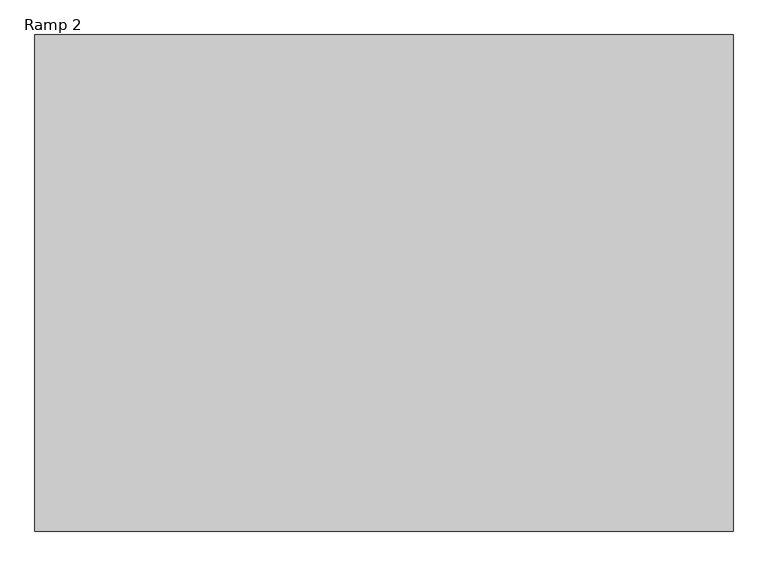
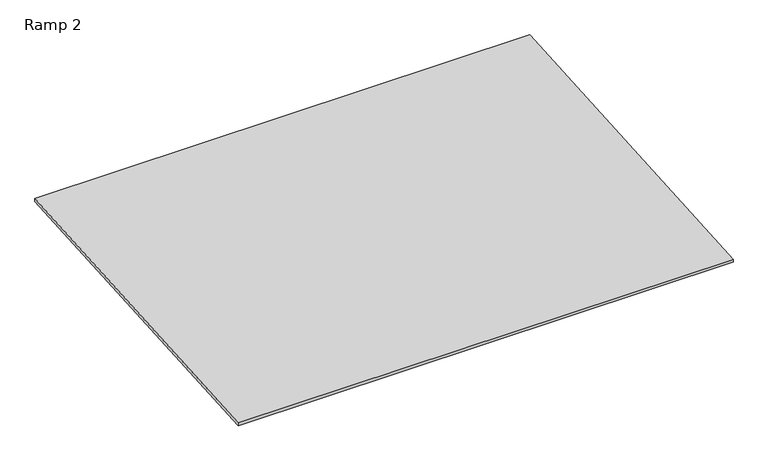
"""IFC4 building model written with IfcOpenShell, lengths in millimetres: ramp geometry, Ramp 2."""

from ifc_helpers import new_model, si_unit, frame, origin, place, context, project, spatial, polyline, outline, extrude, source, transform, mapped, element, save


def ramp_2_3d1851f7(model_context):
    return source(origin(), model_context, "Body", "SweptSolid", [
        extrude(outline(polyline([(-16300.9018845, -914.4), (-7374.0266794, -304.8), (-7374.0266794, -381.1774641), (-16300.9018845, -990.7774641), (-16300.9018845, -914.4)])), frame((-12421.1789065, 0.0, 0.0), z_axis=(1.0, 0.0, 0.0), x_axis=(0.0, 1.0, 0.0)), (0.0, 0.0, 1.0), 12550.837736),
    ])


if __name__ == "__main__":
    model = new_model("IFC4")
    model_context = context("Model", 3, world=origin())
    ifc_project = project(units=[si_unit("LENGTHUNIT", "METRE", prefix="MILLI")], contexts=[model_context])
    site = spatial("IfcSite", under=ifc_project)
    building = spatial("IfcBuilding", under=site)
    placement = place(None, origin())
    ramp_2_shape = ramp_2_3d1851f7(model_context)
    element("IfcRamp", 1, ObjectType="Ramp 2", at=placement, inside=building, context=model_context, shape_type="MappedRepresentation", body=[
        mapped(ramp_2_shape, transform((0.0, 0.0, 0.0), x_axis=(1.0, 0.0, 0.0), y_axis=(0.0, 1.0, 0.0), z_axis=(0.0, 0.0, 1.0))),
    ])
    save(model, "model.ifc")
